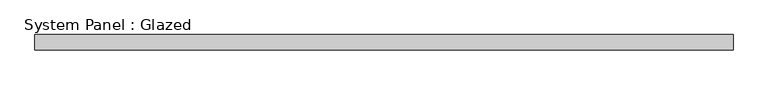
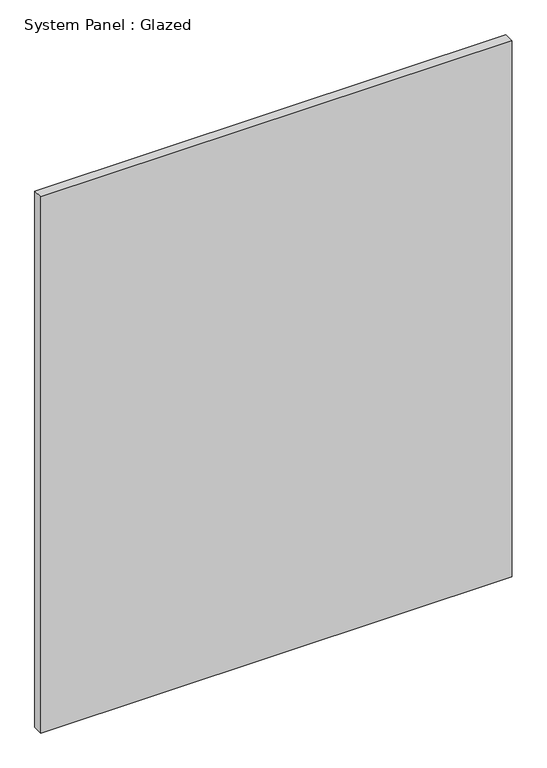
"""IFC4 building model written with IfcOpenShell, lengths in millimetres: plate geometry, System Panel : Glazed."""

from ifc_helpers import new_model, si_unit, origin, origin_with_axes, place, context, project, spatial, polyline, outline, extrude, source, transform, mapped, element, save


def system_panel_glazed_e991d7fc(model_context):
    return source(origin(), model_context, "Body", "SweptSolid", [
        extrude(outline(polyline([(580.39, 19.05), (-580.39, 19.05), (-580.39, 44.45), (580.39, 44.45), (580.39, 19.05)])), origin_with_axes(), (0.0, 0.0, 1.0), 1395.1131867),
    ])


if __name__ == "__main__":
    model = new_model("IFC4")
    model_context = context("Model", 3, world=origin())
    ifc_project = project(units=[si_unit("LENGTHUNIT", "METRE", prefix="MILLI")], contexts=[model_context])
    site = spatial("IfcSite", under=ifc_project)
    building = spatial("IfcBuilding", under=site)
    placement = place(None, origin())
    system_panel_glazed_shape = system_panel_glazed_e991d7fc(model_context)
    element("IfcPlate", 1, ObjectType="System Panel : Glazed", at=placement, inside=building, context=model_context, shape_type="MappedRepresentation", body=[
        mapped(system_panel_glazed_shape, transform((0.0, 0.0, 0.0), x_axis=(1.0, 0.0, 0.0), y_axis=(0.0, 1.0, 0.0), z_axis=(0.0, 0.0, 1.0))),
    ])
    save(model, "model.ifc")

# Revit data of these elements
# Type "System Panel : Glazed"
#   Construction Type Id = "GSP4R"
#   Analytic Construction = "1/8 in Pilkington single glazing"
#   Visual Light Transmittance = 0.9
#   Solar Heat Gain Coefficient = 0.86
#   Heat Transfer Coefficient (U) = 1.18115 BTU/(h·ft²·°F)
#   Define Thermal Properties by = 1
# Element 1 (IfcPlate, "System Panel : Glazed")
#   Materials on its faces: "Glass"
# Materials
#   "Glass": class "Glass", colour RGB 0 128 192, transparency 0.75, Description = "Soda Lime Glass", Cost = 0
